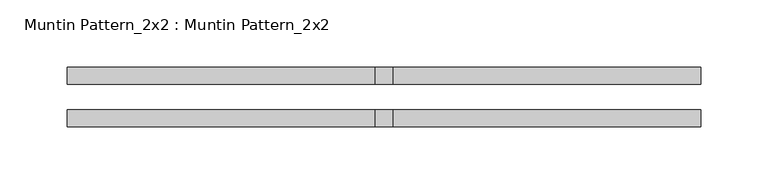
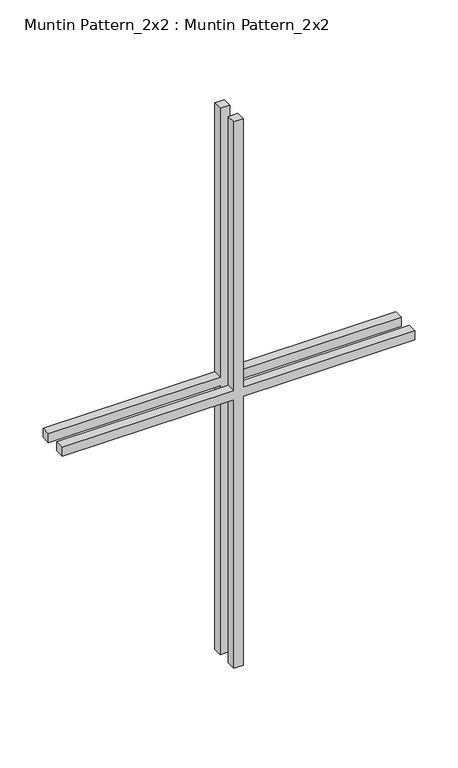
"""IFC4 building model written with IfcOpenShell, lengths in millimetres: proxy geometry, Muntin Pattern_2x2 : Muntin Pattern_2x2."""

from ifc_helpers import new_model, si_unit, frame, origin, place, context, project, spatial, polyline, outline, extrude, source, transform, mapped, element, save


def muntin_pattern_2x2_muntin_pattern_2x2_2357e71d(model_context):
    return source(origin(), model_context, "Body", "SweptSolid", [
        extrude(outline(polyline([(393.7, -6.35), (393.7, -236.5375), (381.0, -236.5375), (381.0, -6.35), (0.0, -6.35), (0.0, 6.35), (381.0, 6.35), (381.0, 236.5375), (393.7, 236.5375), (393.7, 6.35), (774.7, 6.35), (774.7, -6.35), (393.7, -6.35)])), frame((0.0, 9.525, 0.0), z_axis=(0.0, 1.0, 0.0), x_axis=(0.0, 0.0, 1.0)), (0.0, 0.0, 1.0), 12.7),
        extrude(outline(polyline([(393.7, -6.35), (393.7, -236.5375), (381.0, -236.5375), (381.0, -6.35), (0.0, -6.35), (0.0, 6.35), (381.0, 6.35), (381.0, 236.5375), (393.7, 236.5375), (393.7, 6.35), (774.7, 6.35), (774.7, -6.35), (393.7, -6.35)])), frame((0.0, -22.225, 0.0), z_axis=(0.0, 1.0, 0.0), x_axis=(0.0, 0.0, 1.0)), (0.0, 0.0, 1.0), 12.7),
    ])


if __name__ == "__main__":
    model = new_model("IFC4")
    model_context = context("Model", 3, world=origin())
    ifc_project = project(units=[si_unit("LENGTHUNIT", "METRE", prefix="MILLI")], contexts=[model_context])
    site = spatial("IfcSite", under=ifc_project)
    building = spatial("IfcBuilding", under=site)
    placement = place(None, origin())
    muntin_pattern_2x2_muntin_pattern_2x2_shape = muntin_pattern_2x2_muntin_pattern_2x2_2357e71d(model_context)
    element("IfcBuildingElementProxy", 1, Name="Muntin Pattern_2x2 : Muntin Pattern_2x2", ObjectType="Muntin Pattern_2x2 : Muntin Pattern_2x2", at=placement, inside=building, context=model_context, shape_type="MappedRepresentation", body=[
        mapped(muntin_pattern_2x2_muntin_pattern_2x2_shape, transform((0.0, 0.0, 0.0), x_axis=(1.0, 0.0, 0.0), y_axis=(0.0, 1.0, 0.0), z_axis=(0.0, 0.0, 1.0))),
    ])
    save(model, "model.ifc")

# Revit data of these elements
# Type "Muntin Pattern_2x2 : Muntin Pattern_2x2"
#   Width [instance default] = 4' - 0"
#   Thickness = 0' - 0 1/2"
#   Height [instance default] = 4' - 0"
#   Distance = 0' - 0 3/4"
#   Interior Material [instance default] = none
#   Exterior Material [instance default] = none
#   Default Elevation = 0
# Element 1 (IfcBuildingElementProxy, "Muntin Pattern_2x2 : Muntin Pattern_2x2")
#   Width = 1' - 6 5/8"
#   Height = 2' - 6 1/2"
#   Interior Material = Wood - Stained
#   Exterior Material = Clad - White
#   Materials on its faces: "Clad - White", "Wood - Stained"
# Materials
#   "Clad - White": class "Wood", colour RGB 242 242 238, transparency 0, Cost = 0
#   "Wood - Stained": class "Wood", colour RGB 224 178 126, transparency 0, Cost = 0
